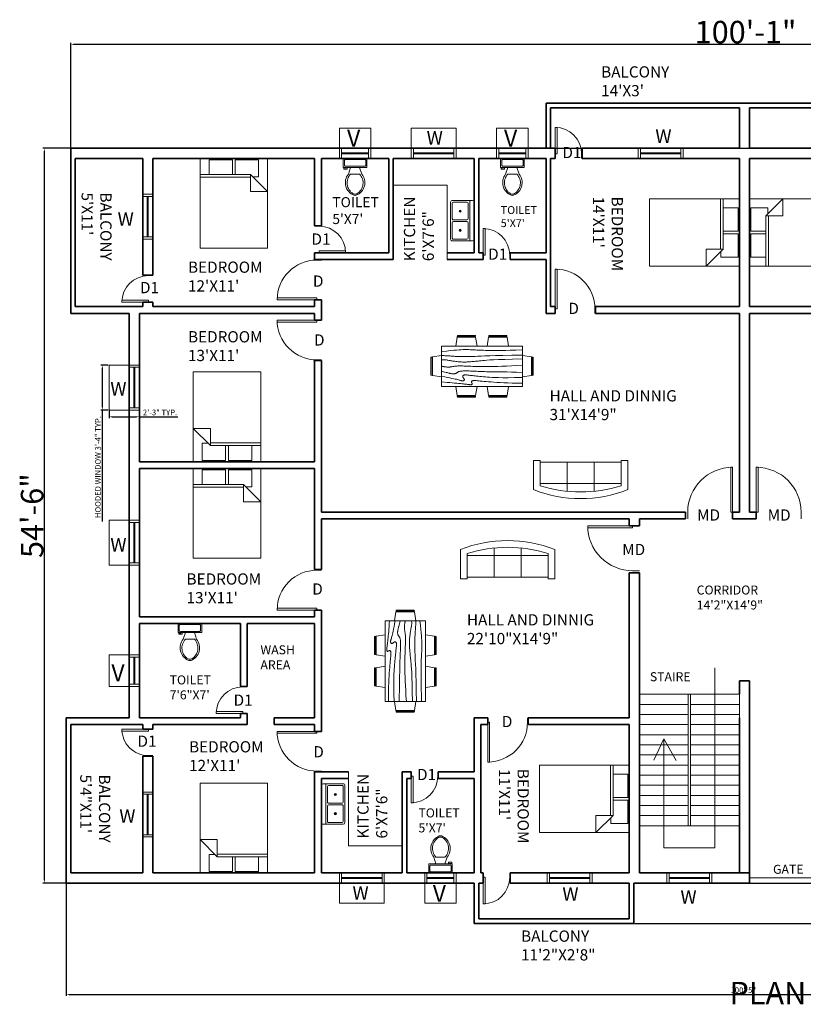
# Model space of a CAD drawing. Units: inches. Extents: x 1662 to 23131, y 1265 to 19127.
# Tile 18 of 26: x 19450 to 20147, y 18251 to 19127. Entities that reach past the tile are written whole.
import ezdxf

# ---------------------------------------------------------------- set-up
doc = ezdxf.new("R2010")
doc.units = ezdxf.units.IN
for name, color, linetype, lineweight in [('A-ANNO-DIMS', 4, 'Continuous', 18), ('A-ANNO-IDEN', 7, 'Continuous', 18), ('A-ANNO-TITL', 7, 'Continuous', 35), ('A-AREA-IDEN', 7, 'Continuous', 18), ('A-DOOR', 3, 'Continuous', 18), ('A-DOOR-GATE', 3, 'Continuous', 18), ('A-FLOR-CASE', 8, 'Continuous', 18), ('A-FLOR-FIXT', 9, 'Continuous', 18), ('A-FLOR-STRS', 7, 'Continuous', 18), ('A-FURN', 8, 'Continuous', 18), ('A-GLAZ', 4, 'Continuous', 18), ('A-WALL', 7, 'Continuous', 35)]:
    doc.layers.add(name, color=color, linetype=linetype, lineweight=lineweight)
doc.styles.get("Standard").update_dxf_attribs({"font": 'arial.ttf'})
doc.dimstyles.new('ISO-25', dxfattribs={"dimtxt": 5, "dimasz": 2.5, "dimexe": 1.25, "dimexo": 0.625, "dimtad": 1, "dimlunit": 3, "dimtxsty": 'Standard', "dimcen": 2.5, "dimadec": 0, "dimazin": 0, "dimtfac": 1, "dimtmove": 0, "dimatfit": 3, "dimfxl": 1, "dimarcsym": 0})

# ---------------------------------------------------------------- blocks, each defined once
blk = doc.blocks.new('Bed - Queen')
for p, q in [((0, -80.00003), (0, 0)), ((0, 0), (59.99999, 0)), ((59.99999, 0), (59.99999, -80.00003)), ((7.99999, -1.2), (28.79998, -1.2)), ((7.99999, -14.4), (7.99999, -1.2)), ((28.79998, -1.2), (28.79998, -14.4)), ((31.19999, -1.2), (51.99999, -1.2)), ((31.19999, -14.4), (31.19999, -1.2)), ((51.99999, -1.2), (51.99999, -16.4)), ((0, -14.4), (44.8, -14.4)), ((44.8, -16.8), (0, -16.8)), ((59.99999, -29.6), (44.8, -14.4)), ((44.8, -14.4), (44.8, -29.6)), ((51.99999, -16.4), (46.79936, -16.4)), ((44.8, -29.6), (59.99999, -29.6)), ((59.99999, -80.00003), (0, -80.00003))]:
    blk.add_line(p, q)
blk = doc.blocks.new('Toilet - top')
for p, q in [((-10, -8.5), (-8, -8.5)), ((-10, -9.5), (-10, -8.5)), ((-8, -8.5), (-8, -8)), ((-7, -8), (-7, -9.5)), ((-4, -8), (-6, -14)), ((4, -8), (6, -14)), ((9.5, -6), (9.5, -2)), ((-7, -9.5), (-10, -9.5)), ((4, -14), (-4, -14))]:
    blk.add_line(p, q)
blk.add_lwpolyline([(10.5, -8), (10.5, 0), (-10.5, 0), (-10.5, -8)], close=True)
for points in [[(-9.5, -2), (-9.5, -6)], [(8.5, -1), (-8.5, -1)], [(-8.5, -7), (8.5, -7)]]:
    blk.add_lwpolyline(points)
for centre, radius, start, end in [((-8.62, -1.88), 0.884, 81.8699, 188.1301), ((-8.62, -6.12), 0.884, 171.8699, 278.1301), ((8.62, -1.88), 0.884, 351.8699, 98.1301), ((8.62, -6.12), 0.884, 261.8699, 8.1301), ((3.52, -21.58), 12.17, 141.46911, 247.97143), ((4.2, -21.82), 11.33, 136.36773, 238.94682), ((-3.52, -21.58), 12.17, 292.02843, 38.53071), ((-4.2, -21.82), 11.33, 301.05301, 43.63209), ((0, -27.88), 4, 245.73182, 294.26817), ((0, -29), 4, 254.86053, 285.13947)]:
    blk.add_arc(centre, radius, start, end)
blk = doc.blocks.new('Sink-double - 36 in top')
for p, q in [((-18, -4), (18, -4)), ((-0.75, -18.5), (-0.75, -6.5)), ((0.75, -6.5), (0.75, -18.5))]:
    blk.add_line(p, q)
for points in [[(-16.5, 0), (16.5, 0)], [(-18, -19.5), (-18, -1.5)], [(-16.5, -18.5), (-16.5, -6.5)], [(-15.5, -5.5), (-1.75, -5.5)], [(1.75, -5.5), (15.5, -5.5)], [(16.5, -6.5), (16.5, -18.5)], [(18, -1.5), (18, -19.5)], [(16.5, -21), (-16.5, -21)], [(-1.75, -19.5), (-15.5, -19.5)], [(15.5, -19.5), (1.75, -19.5)]]:
    blk.add_lwpolyline(points)
for centre, radius in [((-8.5, -12.5), 1), ((-8.5, -12.5), 0.5), ((8.5, -12.5), 1), ((8.5, -12.5), 0.5)]:
    blk.add_circle(centre, radius)
for centre, radius, start, end in [((-16.5, -1.5), 1.5, 90, 180), ((16.5, -1.5), 1.5, 0, 90), ((-15.5, -6.5), 1, 90, 180), ((-1.75, -6.5), 1, 0, 90), ((1.75, -6.5), 1, 90, 180), ((15.5, -6.5), 1, 0, 90), ((-16.5, -19.5), 1.5, 180, 270), ((-15.5, -18.5), 1, 180, 270), ((-1.75, -18.5), 1, 270, 0), ((1.75, -18.5), 1, 180, 270), ((15.5, -18.5), 1, 270, 0), ((16.5, -19.5), 1.5, 270, 0)]:
    blk.add_arc(centre, radius, start, end)
blk = doc.blocks.new('Dining Set - 36 x 72 in.')
for p, q in [((-22, 27.5), (-22.1562, 26.50042)), ((-5.8416, 26.5), (-22.1534, 26.5)), ((-22, 27.5), (-6, 27.5)), ((-5.8437, 26.49966), (-6, 27.5)), ((6, 27.5), (5.8438, 26.50042)), ((22.1584, 26.5), (5.8466, 26.5)), ((6, 27.5), (22, 27.5)), ((22.1563, 26.49966), (22, 27.5)), ((36, 18), (-36, 18)), ((-36, 18), (-36, -18)), ((-22.2343, 26.00059), (-23.4847, 17.99762)), ((-22.2304, 26), (-5.7608, 26)), ((-4.5152, 17.99762), (-5.7655, 25.99926)), ((5.7657, 26.00059), (4.5153, 17.99762)), ((5.7696, 26), (22.2392, 26)), ((23.4848, 17.99762), (22.2345, 25.99926)), ((36, -18), (36, 18)), ((-44.0006, 8.23428), (-35.9976, 9.48474)), ((44.0006, 8.23428), (35.9976, 9.48474)), ((-45.5, 8), (-44.5004, 8.15617)), ((-45.5, 8), (-45.5, -8)), ((-44.5, -8.15843), (-44.5, 8.15338)), ((-44, 8.23041), (-44, -8.23915)), ((44, 8.23041), (44, -8.23915)), ((44.5, -8.15843), (44.5, 8.15338)), ((45.5, 8), (44.5005, 8.15617)), ((45.5, 8), (45.5, -8)), ((-44.4997, -8.15631), (-45.5, -8)), ((-35.9976, -9.48476), (-43.9993, -8.2345)), ((35.9976, -9.48476), (43.9993, -8.2345)), ((44.4997, -8.15631), (45.5, -8)), ((-36, -18), (36, -18)), ((-22.2343, -26.0006), (-23.4847, -17.99762)), ((-22.2304, -26), (-5.7608, -26)), ((-4.5152, -17.99762), (-5.7655, -25.99928)), ((5.7657, -26.0006), (4.5153, -17.99762)), ((5.7696, -26), (22.2392, -26)), ((23.4848, -17.99762), (22.2345, -25.99928)), ((-22, -27.5), (-22.1562, -26.50044)), ((-5.8416, -26.5), (-22.1534, -26.5)), ((-22, -27.5), (-6, -27.5)), ((-5.8437, -26.49967), (-6, -27.5)), ((6, -27.5), (5.8438, -26.50044)), ((22.1584, -26.5), (5.8466, -26.5)), ((6, -27.5), (22, -27.5)), ((22.1563, -26.49967), (22, -27.5))]:
    blk.add_line(p, q)
for points in [[(-36, 15), (-31.1772, 14.97754), (-26.8079, 14.91406), (-22.8538, 14.81543), (-19.276, 14.6875), (-16.0362, 14.53613), (-13.0957, 14.36718), (-10.4159, 14.18652), (-7.9583, 14), (-5.6904, 13.81315), (-3.6035, 13.63021), (-1.6954, 13.45508), (0.0365, 13.29166), (1.5945, 13.14388), (2.9811, 13.01562), (4.1988, 12.9108), (5.25, 12.83333), (6.1393, 12.78613), (6.8802, 12.76823), (7.4883, 12.77767), (7.9792, 12.8125), (8.3685, 12.87077), (8.6719, 12.95052), (8.9049, 13.0498), (9.0833, 13.16666), (9.2205, 13.29899), (9.3216, 13.44401), (9.3895, 13.59879), (9.4271, 13.76041), (9.4373, 13.92594), (9.4232, 14.09245), (9.3875, 14.257), (9.3333, 14.41666), (9.2638, 14.56917), (9.1836, 14.71484), (9.0975, 14.85465), (9.0104, 14.98958), (8.9272, 15.1206), (8.8529, 15.2487), (8.7922, 15.37483), (8.75, 15.5), (8.7305, 15.62467), (8.7344, 15.74739), (8.7617, 15.86621), (8.8125, 15.97916), (8.8867, 16.08431), (8.9844, 16.17968), (9.1055, 16.26334), (9.25, 16.33333), (9.4189, 16.38802), (9.6172, 16.42708), (9.8506, 16.45052), (10.125, 16.45833), (10.4463, 16.45052), (10.8203, 16.42708), (11.2529, 16.38802), (11.75, 16.33333), (12.3184, 16.26318), (12.9694, 16.17838), (13.7151, 16.07991), (14.5677, 15.96875), (15.5395, 15.84586), (16.6426, 15.71224), (17.8893, 15.56884), (19.2917, 15.41666), (20.859, 15.25667), (22.5879, 15.08984), (24.4721, 14.91715), (26.5052, 14.73958), (28.6809, 14.5581), (30.9929, 14.3737), (33.4347, 14.18733), (36, 14)], [(-36, 10), (-28.9766, 10.14274), (-23.1725, 10.20442), (-18.4241, 10.19775), (-14.5677, 10.13541), (-11.4399, 10.03011), (-8.877, 9.89453), (-6.7154, 9.74137), (-4.7917, 9.58333), (-2.9698, 9.43082), (-1.2246, 9.28515), (0.4415, 9.14534), (2.026, 9.01041), (3.5266, 8.87939), (4.9408, 8.7513), (6.266, 8.62516), (7.5, 8.5), (8.6411, 8.37549), (9.6914, 8.2539), (10.6538, 8.13818), (11.5312, 8.03125), (12.3267, 7.93603), (13.043, 7.85547), (13.6831, 7.79248), (14.25, 7.75), (14.7471, 7.7303), (15.1797, 7.73307), (15.5537, 7.75732), (15.875, 7.80208), (16.1494, 7.86637), (16.3828, 7.94922), (16.5811, 8.04964), (16.75, 8.16666), (16.8944, 8.29915), (17.0143, 8.44531), (17.1089, 8.60319), (17.1771, 8.77083), (17.218, 8.94629), (17.2305, 9.1276), (17.2137, 9.31282), (17.1667, 9.5), (17.0895, 9.6875), (16.987, 9.875), (16.8649, 10.0625), (16.7292, 10.25), (16.5856, 10.4375), (16.4401, 10.625), (16.2985, 10.8125), (16.1667, 11), (16.05, 11.18733), (15.9518, 11.3737), (15.8752, 11.5581), (15.8229, 11.73958), (15.798, 11.91715), (15.8034, 12.08984), (15.842, 12.25667), (15.9167, 12.41666), (16.0295, 12.56836), (16.1784, 12.70833), (16.3605, 12.83268), (16.5729, 12.9375), (16.8127, 13.01888), (17.0768, 13.07291), (17.3625, 13.0957), (17.6667, 13.08333), (17.9894, 13.03312), (18.3418, 12.94726), (18.7382, 12.82918), (19.1927, 12.68229), (19.7195, 12.51001), (20.3327, 12.31575), (21.0465, 12.10294), (21.875, 11.875), (22.8357, 11.63354), (23.959, 11.37304), (25.2786, 11.08618), (26.8282, 10.76562), (28.6414, 10.40405), (30.752, 9.99414), (33.1936, 9.52856), (36, 9)], [(-36, 5.5), (-30.7157, 5.3348), (-26.069, 5.20963), (-21.9946, 5.11767), (-18.4271, 5.05208), (-15.3009, 5.00602), (-12.5508, 4.97265), (-10.1112, 4.94515), (-7.9167, 4.91666), (-5.909, 4.88167), (-4.0586, 4.83984), (-2.3429, 4.79215), (-0.7396, 4.73958), (0.7739, 4.6831), (2.22, 4.6237), (3.6213, 4.56233), (5, 4.5), (6.373, 4.43782), (7.7344, 4.3776), (9.0723, 4.32129), (10.375, 4.27083), (11.6309, 4.22819), (12.8281, 4.19531), (13.9551, 4.17415), (15, 4.16666), (15.954, 4.17448), (16.819, 4.19791), (17.6001, 4.23698), (18.3021, 4.29166), (18.9299, 4.36198), (19.4883, 4.44791), (19.9823, 4.54948), (20.4167, 4.66666), (20.7969, 4.79899), (21.1302, 4.94401), (21.4245, 5.09879), (21.6875, 5.26041), (21.9271, 5.42594), (22.1511, 5.59245), (22.3672, 5.757), (22.5834, 5.91666), (22.8065, 6.06868), (23.0404, 6.21093), (23.2879, 6.34147), (23.5521, 6.45833), (23.8358, 6.55957), (24.142, 6.64323), (24.4735, 6.70735), (24.8334, 6.75), (25.2235, 6.76969), (25.642, 6.76692), (26.0858, 6.74267), (26.5521, 6.69791), (27.0379, 6.63362), (27.5404, 6.55078), (28.0565, 6.45036), (28.5834, 6.33333), (29.1242, 6.19987), (29.7071, 6.04687), (30.3661, 5.87044), (31.1354, 5.66666), (32.0493, 5.43164), (33.142, 5.16146), (34.4475, 4.85221), (36, 4.5)], [(-36, -1), (-30.7915, -0.6591), (-26.0195, -0.38216), (-21.6519, -0.16284), (-17.6563, 0.00521), (-14.0005, 0.12833), (-10.6523, 0.21289), (-7.5796, 0.26522), (-4.75, 0.29166), (-2.134, 0.29793), (0.2878, 0.28711), (2.5317, 0.26163), (4.6146, 0.22396), (6.5529, 0.17651), (8.3633, 0.12174), (10.0623, 0.06209), (11.6667, 0), (13.1899, -0.06201), (14.6341, -0.1211), (15.9982, -0.17432), (17.2813, -0.21875), (18.4823, -0.25147), (19.6003, -0.26953), (20.6343, -0.27002), (21.5834, -0.25), (22.4481, -0.20768), (23.2357, -0.14584), (23.9549, -0.06836), (24.6146, 0.02083), (25.2235, 0.11784), (25.7904, 0.21875), (26.3241, 0.31966), (26.8334, 0.41666), (27.3265, 0.50618), (27.8099, 0.58593), (28.2894, 0.65397), (28.7709, 0.70833), (29.2601, 0.74707), (29.763, 0.76823), (30.2855, 0.76985), (30.8334, 0.75), (31.4088, 0.70784), (31.9994, 0.64713), (32.589, 0.57275), (33.1615, 0.48958), (33.7008, 0.4025), (34.1908, 0.3164), (34.6153, 0.23616), (34.9584, 0.16666), (35.2099, 0.11165), (35.3848, 0.07031), (35.504, 0.04069), (35.5886, 0.02083), (35.6594, 0.00879), (35.7377, 0.0026), (35.8442, 0.00032), (36, 0)], [(-36, -6.5), (-27.1843, -6.31267), (-20.084, -6.1263), (-14.469, -5.9419), (-10.1094, -5.76042), (-6.7752, -5.58285), (-4.2363, -5.41016), (-2.2629, -5.24333), (-0.625, -5.08334), (0.8708, -4.93099), (2.2715, -4.78646), (3.5872, -4.64974), (4.8281, -4.52084), (6.0046, -4.39974), (7.127, -4.28646), (8.2053, -4.18099), (9.25, -4.08334), (10.2705, -3.99382), (11.2734, -3.91407), (12.2647, -3.84603), (13.25, -3.79167), (14.2354, -3.75293), (15.2266, -3.73177), (16.2295, -3.73015), (17.25, -3.75), (18.2912, -3.79248), (19.3451, -3.85547), (20.4009, -3.93604), (21.4479, -4.03125), (22.4754, -4.13819), (23.4727, -4.25391), (24.4289, -4.37549), (25.3334, -4.5), (26.1785, -4.62492), (26.9694, -4.74935), (27.7145, -4.87281), (28.4219, -4.99479), (29.1, -5.11483), (29.7572, -5.23242), (30.4016, -5.34709), (31.0417, -5.45834), (31.6837, -5.56437), (32.3262, -5.65821), (32.9658, -5.73153), (33.599, -5.77604), (34.2224, -5.78345), (34.8327, -5.74545), (35.4264, -5.65373), (36, -5.5)], [(-36, -10), (-26.4022, -9.81299), (-18.4675, -9.62891), (-11.9839, -9.45069), (-6.7396, -9.28125), (-2.5226, -9.12354), (0.8789, -8.98047), (3.6769, -8.85498), (6.0833, -8.75), (8.2767, -8.66765), (10.3021, -8.60677), (12.1712, -8.56543), (13.8958, -8.54167), (15.4876, -8.53353), (16.9583, -8.53907), (18.3197, -8.55632), (19.5834, -8.58334), (20.7616, -8.61841), (21.8685, -8.66081), (22.9188, -8.71004), (23.9271, -8.76563), (24.9081, -8.82707), (25.8763, -8.89388), (26.8465, -8.96558), (27.8334, -9.04167), (28.8474, -9.12118), (29.8828, -9.20117), (30.93, -9.27824), (31.9792, -9.34896), (33.0205, -9.40991), (34.0443, -9.45768), (35.0407, -9.48885), (36, -9.5)], [(-36, -14.5), (-30.0881, -14.33513), (-25.0332, -14.21224), (-20.7312, -14.12647), (-17.0781, -14.07292), (-13.97, -14.04671), (-11.3027, -14.04297), (-8.9724, -14.05681), (-6.875, -14.08334), (-4.9224, -14.11833), (-3.0905, -14.16016), (-1.3709, -14.20785), (0.2448, -14.26042), (1.7647, -14.3169), (3.1973, -14.3763), (4.5507, -14.43767), (5.8333, -14.5), (7.0554, -14.5621), (8.235, -14.62175), (9.3922, -14.67652), (10.5469, -14.72396), (11.7192, -14.76164), (12.929, -14.78711), (14.1965, -14.79794), (15.5417, -14.79167), (16.9933, -14.76424), (18.6152, -14.70508), (20.4804, -14.60197), (22.6615, -14.44271), (25.2312, -14.21509), (28.2624, -13.9069), (31.8277, -13.50594), (36, -13)]]:
    blk.add_lwpolyline(points)
blk = doc.blocks.new('Sofa - Roundback 7 ft.')
for p, q in [((-12.00002, -32.4421), (-12.00003, -6.5971)), ((11.99997, -32.4421), (11.99998, -6.5971)), ((-36.000027, -34), (-36.000027, -11.4696)), ((-35.999844, -13.3819), (35.9998, -13.3819)), ((35.99998, -34), (35.99998, -11.4696)), ((-36.000027, -32.4421), (35.99998, -32.4421))]:
    blk.add_line(p, q)
for points in [[(-36.000027, -34), (-42.000027, -34), (-42.000027, -8)], [(41.99998, -8), (41.99998, -34), (35.99998, -34)]]:
    blk.add_lwpolyline(points)
for centre, radius, start, end in [((0, -114.25), 114.25, 68.43141, 111.5686), ((-0.00001, -127.1968), 121.1968, 72.72033, 107.2797)]:
    blk.add_arc(centre, radius, start, end)
blk = doc.blocks.new('*U26')
for p, q in [((0, 0), (0, -100)), ((900, 0), (900, -100))]:
    blk.add_line(p, q)
blk.add_lwpolyline([(0, 0), (0, 900), (43.75, 900), (43.75, 0)], close=True)
blk.add_arc((0, 0), 900, 0, 90)
blk = doc.blocks.new('*U99')
for p, q in [((0, 0), (0, 100)), ((900, 0), (900, 100))]:
    blk.add_line(p, q)
blk.add_lwpolyline([(0, 0), (0, -900), (43.75, -900), (43.75, 0)], close=True)
blk.add_arc((0, 0), 900, 270, 0)
blk = doc.blocks.new('*U102')
for p, q in [((0, 0), (0, 100)), ((900, 0), (900, 100))]:
    blk.add_line(p, q)
blk.add_lwpolyline([(0, 0), (0, -900), (43.75, -900), (43.75, 0)], close=True)
blk.add_arc((0, 0), 900, 270, 0)
blk = doc.blocks.new('*U100')
for p, q in [((-900, 0), (-900, 100)), ((0, 0), (0, 100))]:
    blk.add_line(p, q)
blk.add_lwpolyline([(0, 0), (0, -900), (-43.75, -900), (-43.75, 0)], close=True)
blk.add_arc((0, 0), 900, 180, 270)
blk = doc.blocks.new('*U109')
for p, q in [((0, 0), (0, 100)), ((600, 0), (600, 100))]:
    blk.add_line(p, q)
blk.add_lwpolyline([(0, 0), (0, -600), (43.75, -600), (43.75, 0)], close=True)
blk.add_arc((0, 0), 600, 270, 0)
blk = doc.blocks.new('*U110')
for p, q in [((-600, 0), (-600, 100)), ((0, 0), (0, 100))]:
    blk.add_line(p, q)
blk.add_lwpolyline([(0, 0), (0, -600), (-43.75, -600), (-43.75, 0)], close=True)
blk.add_arc((0, 0), 600, 180, 270)
blk = doc.blocks.new('*U105')
for p, q in [((-600, 0), (-600, -100)), ((0, 0), (0, -100))]:
    blk.add_line(p, q)
blk.add_lwpolyline([(0, 0), (0, 600), (-43.75, 600), (-43.75, 0)], close=True)
blk.add_arc((0, 0), 600, 90, 180)
blk = doc.blocks.new('*U112')
for p, q in [((-600, 0), (-600, 100)), ((0, 0), (0, 100))]:
    blk.add_line(p, q)
blk.add_lwpolyline([(0, 0), (0, -600), (-43.75, -600), (-43.75, 0)], close=True)
blk.add_arc((0, 0), 600, 180, 270)
blk = doc.blocks.new('*U111')
for p, q in [((0, 0), (0, 100)), ((600, 0), (600, 100))]:
    blk.add_line(p, q)
blk.add_lwpolyline([(0, 0), (0, -600), (43.75, -600), (43.75, 0)], close=True)
blk.add_arc((0, 0), 600, 270, 0)
blk = doc.blocks.new('*U10')
for p, q in [((0, 0), (0, -6)), ((40, 0), (40, -6))]:
    blk.add_line(p, q)
blk.add_lwpolyline([(0, 0), (0, 40), (1.75, 40), (1.75, 0)], close=True)
blk.add_arc((0, 0), 40, 0, 90)
blk = doc.blocks.new('*U27')
for p, q in [((0, 0), (0, -6)), ((-40, 0), (-40, -6))]:
    blk.add_line(p, q)
blk.add_lwpolyline([(0, 0), (0, 40), (-1.75, 40), (-1.75, 0)], close=True)
blk.add_arc((0, 0), 40, 90, 180)
blk = doc.blocks.new('*U114')
for p, q in [((0, 0), (0, 6)), ((40, 0), (40, 6))]:
    blk.add_line(p, q)
blk.add_lwpolyline([(0, 0), (0, -40), (1.75, -40), (1.75, 0)], close=True)
blk.add_arc((0, 0), 40, 270, 0)
blk = doc.blocks.new('*U106')
for p, q in [((-600, 0), (-600, 100)), ((0, 0), (0, 100))]:
    blk.add_line(p, q)
blk.add_lwpolyline([(0, 0), (0, -600), (-43.75, -600), (-43.75, 0)], close=True)
blk.add_arc((0, 0), 600, 180, 270)
blk = doc.blocks.new('*D115')
at = {"layer": 'A-ANNO-DIMS', "color": 0, "lineweight": -2, "transparency": 16777216}
for p, q in [((19495.19, 19013.32), (19495.19, 19106.49)), ((19497.69, 19105.24), (20693.69, 19105.24)), ((20696.19, 19013.32), (20696.19, 19106.49))]:
    blk.add_line(p, q, dxfattribs=at)
at = {"layer": 'A-ANNO-DIMS', "color": 0, "transparency": 16777216}
for points in [[(19497.69, 19105.65), (19497.69, 19104.82), (19495.19, 19105.24)], [(20693.69, 19105.65), (20693.69, 19104.82), (20696.19, 19105.24)]]:
    blk.add_solid(points, dxfattribs=at)
at = {"layer": 'Defpoints', "color": 0, "transparency": 16777216}
for p in [(20696.19, 19105.24), (19495.19, 19012.7), (20696.19, 19012.7)]:
    blk.add_point(p, dxfattribs=at)
at = {"layer": 'A-ANNO-DIMS', "color": 0, "transparency": 16777216, "insert": (20095.69, 19116.07), "char_height": 5, "attachment_point": 5}
blk.add_mtext('{\\H4x;100\'-1"}', dxfattribs=at)
blk = doc.blocks.new('*D116')
at = {"layer": 'A-ANNO-DIMS', "color": 0, "lineweight": -2, "transparency": 16777216}
for p, q in [((19494.57, 19012.7), (19470.34, 19012.7)), ((19471.59, 19010.2), (19471.59, 18361.2)), ((19494.57, 18358.7), (19470.34, 18358.7))]:
    blk.add_line(p, q, dxfattribs=at)
at = {"layer": 'A-ANNO-DIMS', "color": 0, "transparency": 16777216}
for points in [[(19471.17, 19010.2), (19472, 19010.2), (19471.59, 19012.7)], [(19471.17, 18361.2), (19472, 18361.2), (19471.59, 18358.7)]]:
    blk.add_solid(points, dxfattribs=at)
at = {"layer": 'Defpoints', "color": 0, "transparency": 16777216}
for p in [(19495.19, 19012.7), (19471.59, 18358.7), (19495.19, 18358.7)]:
    blk.add_point(p, dxfattribs=at)
at = {"layer": 'A-ANNO-DIMS', "color": 0, "transparency": 16777216, "insert": (19460.75, 18685.7), "char_height": 5, "attachment_point": 5, "rotation": 90}
blk.add_mtext('{\\H4x;54\'-6"}', dxfattribs=at)
blk = doc.blocks.new('WIN-36-J9X2')
for p, q in [((0, 0), (0, 9)), ((2, 0), (2, 9)), ((38, 0), (38, 9)), ((40, 0), (40, 9)), ((38, 5), (2, 5)), ((38, 4.5), (2, 4.5)), ((38, 4), (2, 4))]:
    blk.add_line(p, q)
blk = doc.blocks.new('WIN-36-J9X2-HOOD')
for p, q in [((0, 27), (0, 18)), ((2, 27), (2, 18)), ((38, 27), (38, 18)), ((40, 27), (40, 18)), ((0, 18), (0, 0)), ((2, 23), (38, 23)), ((2, 22.5), (38, 22.5)), ((2, 22), (38, 22)), ((40, 0), (40, 18)), ((0, 0), (40, 0))]:
    blk.add_line(p, q)
blk = doc.blocks.new('VENT-24-J9X2-HOOD')
for p, q in [((0, 18), (0, 27)), ((2, 18), (2, 27)), ((26, 18), (26, 27)), ((28, 18), (28, 27)), ((0, 18), (0, 0)), ((26, 23), (2, 23)), ((26, 22.5), (2, 22.5)), ((26, 22), (2, 22)), ((28, 0), (28, 18)), ((0, 0), (28, 0))]:
    blk.add_line(p, q)
blk = doc.blocks.new('*D173')
at = {"layer": 'A-ANNO-DIMS', "color": 0, "lineweight": -2, "transparency": 16777216}
for p, q in [((19528.57, 18819.7), (19521.94, 18819.7)), ((19523.19, 18817.2), (19523.19, 18782.2)), ((19528.57, 18779.7), (19521.94, 18779.7)), ((19523.19, 18779.7), (19523.19, 18680.55))]:
    blk.add_line(p, q, dxfattribs=at)
at = {"layer": 'A-ANNO-DIMS', "color": 0, "transparency": 16777216}
for points in [[(19522.78, 18817.2), (19523.61, 18817.2), (19523.19, 18819.7)], [(19522.78, 18782.2), (19523.61, 18782.2), (19523.19, 18779.7)]]:
    blk.add_solid(points, dxfattribs=at)
at = {"layer": 'Defpoints', "color": 0, "transparency": 16777216}
for p in [(19529.19, 18819.7), (19523.19, 18779.7), (19529.19, 18779.7)]:
    blk.add_point(p, dxfattribs=at)
at = {"layer": 'A-ANNO-DIMS', "color": 0, "transparency": 16777216, "insert": (19519.98, 18728.87), "char_height": 5, "attachment_point": 5, "rotation": 90}
blk.add_mtext('HOODED WINDOW 3\'-4" TYP.', dxfattribs=at)
blk = doc.blocks.new('*D174')
at = {"layer": 'A-ANNO-DIMS', "color": 0, "lineweight": -2, "transparency": 16777216}
for p, q in [((19529.19, 18779.07), (19529.19, 18772.45)), ((19531.69, 18773.7), (19553.69, 18773.7)), ((19556.19, 18779.07), (19556.19, 18772.45)), ((19556.19, 18773.7), (19590.51, 18773.7))]:
    blk.add_line(p, q, dxfattribs=at)
at = {"layer": 'A-ANNO-DIMS', "color": 0, "transparency": 16777216}
for points in [[(19531.69, 18774.11), (19531.69, 18773.28), (19529.19, 18773.7)], [(19553.69, 18774.11), (19553.69, 18773.28), (19556.19, 18773.7)]]:
    blk.add_solid(points, dxfattribs=at)
at = {"layer": 'Defpoints', "color": 0, "transparency": 16777216}
for p in [(19529.19, 18779.7), (19556.19, 18779.7), (19556.19, 18773.7)]:
    blk.add_point(p, dxfattribs=at)
at = {"layer": 'A-ANNO-DIMS', "color": 0, "transparency": 16777216, "insert": (19574.6, 18776.88), "char_height": 5, "attachment_point": 5}
blk.add_mtext('2\'-3" TYP.', dxfattribs=at)
blk = doc.blocks.new('*D251')
at = {"layer": 'A-ANNO-DIMS', "color": 0, "lineweight": -2, "transparency": 16777216}
for p, q in [((19491.19, 18358.07), (19491.19, 18258.3)), ((20696.19, 18358.07), (20696.19, 18258.3)), ((19493.69, 18259.55), (20693.69, 18259.55))]:
    blk.add_line(p, q, dxfattribs=at)
at = {"layer": 'A-ANNO-DIMS', "color": 0, "transparency": 16777216}
for points in [[(19493.69, 18259.96), (19493.69, 18259.13), (19491.19, 18259.55)], [(20693.69, 18259.96), (20693.69, 18259.13), (20696.19, 18259.55)]]:
    blk.add_solid(points, dxfattribs=at)
at = {"layer": 'Defpoints', "color": 0, "transparency": 16777216}
for p in [(19491.19, 18358.7), (20696.19, 18358.7), (20696.19, 18259.55)]:
    blk.add_point(p, dxfattribs=at)
at = {"layer": 'A-ANNO-DIMS', "color": 0, "transparency": 16777216, "insert": (20093.69, 18262.72), "char_height": 5, "attachment_point": 5}
blk.add_mtext('100\'-5"', dxfattribs=at)
blk = doc.blocks.new('*D252')
at = {"layer": 'A-ANNO-DIMS', "color": 0, "lineweight": -2, "transparency": 16777216}
for p, q in [((19918.82, 19052.7), (20760.59, 19052.7)), ((20759.34, 19015.2), (20759.34, 19050.2)), ((19918.82, 19012.7), (20760.59, 19012.7))]:
    blk.add_line(p, q, dxfattribs=at)
at = {"layer": 'A-ANNO-DIMS', "color": 0, "transparency": 16777216}
for points in [[(20758.93, 19050.2), (20759.76, 19050.2), (20759.34, 19052.7)], [(20758.93, 19015.2), (20759.76, 19015.2), (20759.34, 19012.7)]]:
    blk.add_solid(points, dxfattribs=at)
at = {"layer": 'Defpoints', "color": 0, "transparency": 16777216}
for p in [(19918.19, 19052.7), (20759.34, 19052.7), (19918.19, 19012.7)]:
    blk.add_point(p, dxfattribs=at)
at = {"layer": 'A-ANNO-DIMS', "color": 0, "transparency": 16777216, "insert": (20756.16, 19032.7), "char_height": 5, "attachment_point": 5, "rotation": 90}
blk.add_mtext('3\'-4"', dxfattribs=at)
blk = doc.blocks.new('*D253')
at = {"layer": 'A-ANNO-DIMS', "color": 0, "lineweight": -2, "transparency": 16777216}
for p, q in [((19996.82, 18358.7), (20760.59, 18358.7)), ((20759.34, 18325.2), (20759.34, 18356.2)), ((19996.82, 18322.7), (20760.59, 18322.7))]:
    blk.add_line(p, q, dxfattribs=at)
at = {"layer": 'A-ANNO-DIMS', "color": 0, "transparency": 16777216}
for points in [[(20758.93, 18356.2), (20759.76, 18356.2), (20759.34, 18358.7)], [(20758.93, 18325.2), (20759.76, 18325.2), (20759.34, 18322.7)]]:
    blk.add_solid(points, dxfattribs=at)
at = {"layer": 'Defpoints', "color": 0, "transparency": 16777216}
for p in [(19996.19, 18358.7), (20759.34, 18358.7), (19996.19, 18322.7)]:
    blk.add_point(p, dxfattribs=at)
at = {"layer": 'A-ANNO-DIMS', "color": 0, "transparency": 16777216, "insert": (20756.16, 18340.7), "char_height": 5, "attachment_point": 5, "rotation": 90}
blk.add_mtext('3\'-0"', dxfattribs=at)

msp = doc.modelspace()

# ---------------------------------------------------------------- linework, layer by layer
at = {"layer": 'A-DOOR-GATE'}
msp.add_line((20099.192, 18363.196), (20168.192, 18363.196), dxfattribs=at)
at = {"layer": 'A-FLOR-CASE'}
for p, q in [((19782.192, 18979.696), (19830.192, 18979.696)), ((19830.192, 18913.696), (19830.192, 18979.696)), ((19742.192, 18391.696), (19742.192, 18457.696)), ((19742.192, 18391.696), (19790.192, 18391.696))]:
    msp.add_line(p, q, dxfattribs=at)
at = {"layer": 'A-FLOR-STRS'}
for p, q in [((20068.442, 18550.107), (20068.442, 18390.107)), ((20001.192, 18526.696), (20090.192, 18526.696)), ((20044.692, 18409.696), (20044.692, 18526.696)), ((20046.692, 18409.696), (20046.692, 18526.696)), ((20090.192, 18505.696), (20090.192, 18526.696)), ((20001.192, 18517.696), (20044.692, 18517.696)), ((20046.692, 18517.696), (20090.192, 18517.696)), ((20001.192, 18508.696), (20044.692, 18508.696)), ((20046.692, 18508.696), (20090.192, 18508.696)), ((20001.192, 18499.696), (20044.692, 18499.696)), ((20046.692, 18499.696), (20090.192, 18499.696)), ((20001.192, 18490.696), (20044.692, 18490.696)), ((20022.942, 18486.908), (20013.925, 18467.991)), ((20022.942, 18390.107), (20022.942, 18486.908)), ((20022.942, 18486.908), (20033.987, 18467.711)), ((20046.692, 18490.696), (20090.192, 18490.696)), ((20001.192, 18481.696), (20044.692, 18481.696)), ((20046.692, 18481.696), (20090.192, 18481.696)), ((20001.192, 18472.696), (20044.692, 18472.696)), ((20046.692, 18472.696), (20090.192, 18472.696)), ((20001.192, 18463.696), (20044.692, 18463.696)), ((20046.692, 18463.696), (20090.192, 18463.696)), ((20001.192, 18454.696), (20044.692, 18454.696)), ((20046.692, 18454.696), (20090.192, 18454.696)), ((20001.192, 18445.696), (20044.692, 18445.696)), ((20046.692, 18445.696), (20090.192, 18445.696)), ((20001.192, 18436.696), (20044.692, 18436.696)), ((20046.692, 18436.696), (20090.192, 18436.696)), ((20001.192, 18427.696), (20044.692, 18427.696)), ((20046.692, 18427.696), (20090.192, 18427.696)), ((20001.192, 18418.696), (20044.692, 18418.696)), ((20046.692, 18418.696), (20090.192, 18418.696)), ((20001.192, 18409.696), (20090.192, 18409.696)), ((20068.442, 18390.107), (20022.942, 18390.107))]:
    msp.add_line(p, q, dxfattribs=at)
at = {"layer": 'A-WALL'}
for p, q in [((19918.192, 19012.696), (19918.192, 19052.696)), ((19918.192, 19052.696), (20271.192, 19052.696)), ((19922.192, 19012.696), (19922.192, 19048.696)), ((19922.192, 19048.696), (20090.192, 19048.696)), ((20090.192, 19012.696), (20090.192, 19048.696)), ((20099.192, 19012.696), (20099.192, 19048.696)), ((20099.192, 19048.696), (20267.192, 19048.696)), ((19495.192, 18865.696), (19495.192, 19012.696)), ((19495.192, 19012.696), (19926.192, 19012.696)), ((19926.192, 19003.696), (19926.192, 19012.696)), ((19950.192, 19003.696), (19950.192, 19012.696)), ((19950.192, 19012.696), (20090.192, 19012.696)), ((20099.192, 19012.696), (20239.192, 19012.696)), ((19499.192, 19003.696), (19559.192, 19003.696)), ((19499.192, 18871.696), (19499.192, 19003.696)), ((19559.192, 18899.696), (19559.192, 19003.696)), ((19568.192, 18899.696), (19568.192, 19003.696)), ((19568.192, 19003.696), (19712.192, 19003.696)), ((19712.192, 18943.696), (19712.192, 19003.696)), ((19718.192, 18943.696), (19718.192, 19003.696)), ((19718.192, 19003.696), (19778.192, 19003.696)), ((19778.192, 18919.696), (19778.192, 19003.696)), ((19782.192, 18913.696), (19782.192, 19003.696)), ((19782.192, 19003.696), (19854.192, 19003.696)), ((19854.192, 18919.696), (19854.192, 19003.696)), ((19858.192, 18919.696), (19858.192, 19003.696)), ((19858.192, 19003.696), (19918.192, 19003.696)), ((19918.192, 18919.696), (19918.192, 19003.696)), ((19922.192, 18871.696), (19922.192, 19003.696)), ((19922.192, 19003.696), (19926.192, 19003.696)), ((19950.192, 19003.696), (20090.192, 19003.696)), ((20090.192, 18871.696), (20090.192, 19003.696)), ((20099.192, 19003.696), (20239.192, 19003.696)), ((20099.192, 18871.696), (20099.192, 19003.696)), ((19854.192, 18948.185), (19854.192, 18948.185)), ((19712.192, 18943.696), (19718.192, 18943.696)), ((19712.192, 18919.696), (19778.192, 18919.696)), ((19712.192, 18913.696), (19712.192, 18919.696)), ((19712.192, 18913.696), (19782.192, 18913.696)), ((19830.192, 18919.696), (19854.192, 18919.696)), ((19830.192, 18913.696), (19862.192, 18913.696)), ((19858.192, 18919.696), (19862.192, 18919.696)), ((19862.192, 18913.696), (19862.192, 18919.696)), ((19886.192, 18913.696), (19886.192, 18919.696)), ((19886.192, 18919.696), (19918.192, 18919.696)), ((19886.192, 18913.696), (19918.192, 18913.696)), ((19918.192, 18865.696), (19918.192, 18913.696)), ((19559.192, 18899.696), (19568.192, 18899.696)), ((19712.192, 18877.696), (19718.192, 18877.696)), ((19712.192, 18871.696), (19712.192, 18877.696)), ((19718.192, 18859.696), (19718.192, 18877.696)), ((19499.192, 18871.696), (19559.192, 18871.696)), ((19559.192, 18871.696), (19559.192, 18875.696)), ((19559.192, 18875.696), (19568.192, 18875.696)), ((19568.192, 18871.696), (19568.192, 18875.696)), ((19568.192, 18871.696), (19712.192, 18871.696)), ((19922.192, 18871.696), (19926.192, 18871.696)), ((19926.192, 18865.696), (19926.192, 18871.696)), ((19962.192, 18865.696), (19962.192, 18871.696)), ((19962.192, 18871.696), (20090.192, 18871.696)), ((20099.192, 18871.696), (20227.192, 18871.696)), ((19495.192, 18865.696), (19547.192, 18865.696)), ((19547.192, 18505.696), (19547.192, 18865.696)), ((19556.192, 18865.696), (19712.192, 18865.696)), ((19556.192, 18733.696), (19556.192, 18865.696)), ((19712.192, 18859.696), (19712.192, 18865.696)), ((19718.192, 18859.696), (19712.192, 18859.696)), ((19918.192, 18865.696), (19926.192, 18865.696)), ((19962.192, 18865.696), (20090.192, 18865.696)), ((20090.192, 18688.696), (20090.192, 18865.696)), ((20099.192, 18688.696), (20099.192, 18865.696)), ((20099.192, 18865.696), (20227.192, 18865.696)), ((19718.192, 18823.696), (19712.192, 18823.696)), ((19712.192, 18733.696), (19712.192, 18823.696)), ((19718.192, 18688.696), (19718.192, 18823.696)), ((19556.192, 18733.696), (19712.192, 18733.696)), ((19556.192, 18727.696), (19712.192, 18727.696)), ((19556.192, 18595.696), (19556.192, 18727.696)), ((19712.192, 18637.696), (19712.192, 18727.696)), ((19718.192, 18688.696), (20042.192, 18688.696)), ((20042.192, 18682.696), (20042.192, 18688.696)), ((20084.192, 18682.696), (20084.192, 18688.696)), ((20084.192, 18688.696), (20090.192, 18688.696)), ((20099.192, 18688.696), (20105.192, 18688.696)), ((20105.192, 18682.696), (20105.192, 18688.696)), ((19718.192, 18682.696), (19992.192, 18682.696)), ((19718.192, 18637.696), (19718.192, 18682.696)), ((19992.192, 18676.696), (19992.192, 18682.696)), ((19992.192, 18676.696), (20001.192, 18676.696)), ((20001.192, 18676.696), (20001.192, 18682.696)), ((20001.192, 18682.696), (20042.192, 18682.696)), ((20084.192, 18682.696), (20105.192, 18682.696)), ((19712.192, 18637.696), (19718.192, 18637.696)), ((19992.192, 18505.696), (19992.192, 18634.696)), ((19992.192, 18634.696), (20001.192, 18634.696)), ((20001.192, 18367.696), (20001.192, 18634.696)), ((19712.192, 18601.696), (19718.192, 18601.696)), ((19712.192, 18595.696), (19712.192, 18601.696)), ((19718.192, 18493.696), (19718.192, 18601.696)), ((19556.192, 18595.696), (19712.192, 18595.696)), ((19556.192, 18505.696), (19556.192, 18589.696)), ((19556.192, 18589.696), (19646.192, 18589.696)), ((19646.192, 18533.696), (19646.192, 18589.696)), ((19652.192, 18533.696), (19652.192, 18589.696)), ((19652.192, 18589.696), (19712.192, 18589.696)), ((19712.192, 18505.696), (19712.192, 18589.696)), ((20090.192, 18526.696), (20090.192, 18538.696)), ((20090.192, 18538.696), (20099.192, 18538.696)), ((20099.192, 18538.696), (20099.192, 18499.696)), ((19646.192, 18533.696), (19652.192, 18533.696)), ((19646.192, 18505.696), (19646.192, 18509.696)), ((19646.192, 18509.696), (19652.192, 18509.696)), ((19652.192, 18499.696), (19652.192, 18509.696)), ((19491.192, 18505.696), (19547.192, 18505.696)), ((19491.192, 18505.696), (19491.192, 18358.696)), ((19556.192, 18505.696), (19646.192, 18505.696)), ((19676.192, 18499.696), (19676.192, 18505.696)), ((19676.192, 18505.696), (19712.192, 18505.696)), ((19854.192, 18505.696), (19866.192, 18505.696)), ((19854.192, 18457.696), (19854.192, 18505.696)), ((19866.192, 18499.696), (19866.192, 18505.696)), ((19902.192, 18499.696), (19902.192, 18505.696)), ((19902.192, 18505.696), (19992.192, 18505.696)), ((20090.192, 18367.696), (20090.192, 18505.696)), ((19495.192, 18499.696), (19559.192, 18499.696)), ((19495.192, 18499.696), (19495.192, 18367.696)), ((19559.192, 18499.696), (19559.192, 18495.696)), ((19559.192, 18495.696), (19568.192, 18495.696)), ((19568.192, 18499.696), (19568.192, 18495.696)), ((19568.192, 18499.696), (19652.192, 18499.696)), ((19676.192, 18499.696), (19712.192, 18499.696)), ((19712.192, 18493.696), (19712.192, 18499.696)), ((19712.192, 18493.696), (19718.192, 18493.696)), ((19860.192, 18367.696), (19860.192, 18499.696)), ((19860.192, 18499.696), (19866.192, 18499.696)), ((19902.192, 18499.696), (19992.192, 18499.696)), ((19992.192, 18367.696), (19992.192, 18499.696)), ((20099.192, 18421.696), (20099.192, 18499.696)), ((19559.192, 18471.696), (19568.192, 18471.696)), ((19559.192, 18471.696), (19559.192, 18367.696)), ((19568.192, 18471.696), (19568.192, 18367.696)), ((19712.192, 18367.696), (19712.192, 18457.696)), ((19712.192, 18457.696), (19742.192, 18457.696)), ((19790.192, 18367.696), (19790.192, 18457.696)), ((19790.192, 18457.696), (19798.192, 18457.696)), ((19798.192, 18451.696), (19798.192, 18457.696)), ((19822.192, 18451.696), (19822.192, 18457.696)), ((19822.192, 18457.696), (19854.192, 18457.696)), ((19718.192, 18367.696), (19718.192, 18451.696)), ((19718.192, 18451.696), (19742.192, 18451.696)), ((19794.192, 18367.696), (19794.192, 18451.696)), ((19794.192, 18451.696), (19798.192, 18451.696)), ((19822.192, 18451.696), (19854.192, 18451.696)), ((19854.192, 18367.696), (19854.192, 18451.696)), ((20099.192, 18358.696), (20099.192, 18421.696)), ((19495.192, 18367.696), (19559.192, 18367.696)), ((19568.192, 18367.696), (19712.192, 18367.696)), ((19718.192, 18367.696), (19790.192, 18367.696)), ((19794.192, 18367.696), (19854.192, 18367.696)), ((19860.192, 18367.696), (19862.192, 18367.696)), ((19862.192, 18367.696), (19862.192, 18358.696)), ((19886.192, 18367.696), (19886.192, 18358.696)), ((19886.192, 18367.696), (19992.192, 18367.696)), ((20001.192, 18367.696), (20099.192, 18367.696)), ((19491.192, 18358.696), (19854.192, 18358.696)), ((19854.192, 18358.696), (19854.192, 18322.696)), ((19858.192, 18358.696), (19858.192, 18326.696)), ((19858.192, 18358.696), (19862.192, 18358.696)), ((19886.192, 18358.696), (19992.192, 18358.696)), ((19992.192, 18358.696), (19992.192, 18326.696)), ((19996.192, 18358.696), (20099.192, 18358.696)), ((19996.192, 18358.696), (19996.192, 18322.696)), ((19996.192, 18358.696), (20099.192, 18358.696)), ((19858.192, 18326.696), (19992.192, 18326.696)), ((19854.192, 18322.696), (19996.192, 18322.696))]:
    msp.add_line(p, q, dxfattribs=at)

# ---------------------------------------------------------------- block references
at = {"layer": 'A-DOOR', "xscale": 0.0393700787401575, "yscale": 0.0393700787401575, "zscale": 0.0393700787401575}
for name, p, rotation in [('*U110', (19926.192, 19007.633), 180), ('*U105', (19716.129, 18919.696), 270), ('*U110', (19862.192, 18917.633), 180), ('*U100', (19714.255, 18877.696), 270), ('*U106', (19564.255, 18875.696), 270), ('*U102', (19714.255, 18859.696), 270), ('*U100', (19714.255, 18601.696), 270), ('*U112', (19648.255, 18509.696), 270), ('*U111', (19564.255, 18495.696), 270), ('*U102', (19714.255, 18493.696), 270)]:
    msp.add_blockref(name, p, dxfattribs=dict(at, rotation=rotation))
for name, p in [('*U26', (19926.192, 18869.633)), ('*U99', (19866.192, 18501.759)), ('*U109', (19798.192, 18453.759)), ('*U109', (19862.192, 18363.759))]:
    msp.add_blockref(name, p, dxfattribs=at)
at = {"layer": 'A-DOOR'}
for name, p in [('*U27', (20084.192, 18688.696)), ('*U10', (20105.192, 18688.696))]:
    msp.add_blockref(name, p, dxfattribs=at)
at = {"layer": 'A-DOOR', "rotation": 270}
msp.add_blockref('*U114', (19995.192, 18676.696), dxfattribs=at)
at = {"layer": 'A-FLOR-FIXT'}
for p in [(19748.192, 19003.696), (19888.192, 19003.696), (19601.192, 18589.696)]:
    msp.add_blockref('Toilet - top', p, dxfattribs=at)
for name, p, rotation in [('Sink-double - 36 in top', (19854.192, 18948.185), 270), ('Sink-double - 36 in top', (19718.192, 18428.976), 89.99999999999999), ('Toilet - top', (19824.192, 18367.696), 180)]:
    msp.add_blockref(name, p, dxfattribs=dict(at, rotation=rotation))
at = {"layer": 'A-FURN'}
for name, p in [('Bed - Queen', (19610.192, 19003.696)), ('Bed - Queen', (19604.192, 18727.696)), ('Sofa - Roundback 7 ft.', (19883.918, 18663.493))]:
    msp.add_blockref(name, p, dxfattribs=at)
for name, p, rotation in [('Bed - Queen', (20090.192, 18967.696), 270), ('Bed - Queen', (20099.192, 18907.696), 89.99999999999999), ('Dining Set - 36 x 72 in.', (19861.233, 18818.657), 180), ('Bed - Queen', (19664.192, 18733.696), 180), ('Sofa - Roundback 7 ft.', (19948.928, 18700.835), 180), ('Dining Set - 36 x 72 in.', (19792.827, 18556.13), 89.99999999999996), ('Bed - Queen', (19992.192, 18463.696), 270), ('Bed - Queen', (19670.192, 18367.696), 180)]:
    msp.add_blockref(name, p, dxfattribs=dict(at, rotation=rotation))
at = {"layer": 'A-GLAZ'}
for name, p, rotation in [('VENT-24-J9X2-HOOD', (19762.193, 19030.696), 180), ('WIN-36-J9X2-HOOD', (19838.193, 19030.696), 180), ('VENT-24-J9X2-HOOD', (19902.193, 19030.696), 180), ('WIN-36-J9X2', (19568.192, 18931.696), 90), ('WIN-36-J9X2-HOOD', (19529.192, 18819.697), 270.0000000000059), ('WIN-36-J9X2-HOOD', (19529.192, 18681.697), 270.0000000000059), ('VENT-24-J9X2-HOOD', (19529.192, 18561.697), 270.0000000000246), ('WIN-36-J9X2', (19568.192, 18399.696), 90)]:
    msp.add_blockref(name, p, dxfattribs=dict(at, rotation=rotation))
for name, p in [('WIN-36-J9X2', (20000.192, 19003.696)), ('WIN-36-J9X2-HOOD', (19734.192, 18340.696)), ('VENT-24-J9X2-HOOD', (19810.192, 18340.696)), ('WIN-36-J9X2', (19919.192, 18358.696)), ('WIN-36-J9X2', (20025.692, 18358.696))]:
    msp.add_blockref(name, p, dxfattribs=at)

# ---------------------------------------------------------------- texts
at = {"layer": 'A-ANNO-IDEN', "attachment_point": 1}
for s, width, heights, insert, char_height in [('V', 1142.59551, [20], (19741.017, 19029.237), 15), ('W', 471.52273, [28.462], (19811.874, 19027.97), 12), ('V', 1142.59551, [20], (19880.713, 19029.212), 15), ('W', 471.52273, [28.462], (20015.415, 19029.436), 12), ('D1', 1142.59551, [20], (19932.7, 19013.862), 10), ('W', 471.52273, [28.462], (19536.857, 18955.643), 12), ('D1', 1142.59551, [20], (19709.394, 18936.834), 10), ('D1', 1142.59551, [20], (19866.609, 18923.44), 10), ('D', 1142.59551, [0], (19710.667, 18899.443), 10), ('D1', 1142.59551, [20], (19556.76, 18893.665), 10), ('D', 1142.59551, [0], (19937.99, 18875.136), 10), ('D', 1142.59551, [0], (19711.629, 18847.034), 10), ('W', 471.52273, [28.462], (19530.373, 18804.603), 12), ('MD', 1142.59551, [0], (20052.555, 18691.252), 10), ('MD', 1142.59551, [0], (20115.338, 18691.252), 10), ('W', 471.52273, [28.462], (19530.398, 18665.683), 12), ('MD', 1142.59551, [0], (19985.918, 18660.547), 10), ('D', 1142.59551, [0], (19710.071, 18625.37), 10), ('V', 1142.59551, [20], (19531.286, 18553.338), 15), ('D1', 1142.59551, [20], (19640.069, 18526.478), 10), ('D', 1142.59551, [0], (19878.785, 18507.433), 10), ('D1', 1142.59551, [20], (19554.503, 18489.945), 10), ('D', 1142.59551, [0], (19711.004, 18480.517), 10), ('D1', 1142.59551, [20], (19803.333, 18460.266), 10), ('W', 471.52273, [28.462], (19538.343, 18424.358), 12), ('W', 471.52273, [28.462], (19745.874, 18355.859), 12), ('V', 1142.59551, [20], (19817.337, 18357.074), 15), ('W', 471.52273, [28.462], (19932.677, 18354.879), 12), ('W', 471.52273, [28.462], (20037.753, 18352.273), 12)]:
    msp.add_mtext_dynamic_manual_height_columns(s, width=width, gutter_width=12.5, heights=heights, dxfattribs=dict(at, insert=insert, char_height=char_height))
at = {"layer": 'A-ANNO-TITL', "insert": (20081.333, 18270.744), "char_height": 20, "attachment_point": 1}
msp.add_mtext_dynamic_manual_height_columns('PLAN', width=1142.59551, gutter_width=12.5, heights=[0], dxfattribs=at)
at = {"layer": 'A-AREA-IDEN', "attachment_point": 1}
for s, insert, char_height in [("BALCONY\\P14'X3'", (19967.174, 19085.618), 10), ("TOILET\\P5'X7'", (19727.961, 18969.205), 9), ("TOILET\\P5'X7'", (19877.849, 18961.167), 7), ("BEDROOM\\P12'X11'", (19599.474, 18911.829), 10), ("BEDROOM\\P13'X11'", (19599.474, 18849.889), 10), ('HALL AND DINNIG\\P31\'X14\'9"', (19921.272, 18797.353), 10), ("BEDROOM\\P13'X11'", (19598.183, 18634.313), 10), ('CORRIDOR\\P14\'2"X14\'9"', (20052.179, 18623.491), 8), ('HALL AND DINNIG\\P22\'10"X14\'9"', (19847.691, 18597.959), 10), ('WASH \\PAREA', (19663.957, 18570.254), 8), ('STAIRE', (20010.539, 18546.311), 8), ('TOILET\\P7\'6"X7\'', (19583.157, 18543.472), 8), ("BEDROOM\\P12'X11'", (19600.428, 18484.954), 10), ("TOILET\\P5'X7'", (19804.593, 18425.097), 8), ('GATE', (20120.172, 18374.916), 8), ('BALCONY\\P11\'2"X2\'8"', (19895.902, 18316.449), 10)]:
    msp.add_mtext_dynamic_manual_height_columns(s, width=1142.59551, gutter_width=12.5, heights=[277.772], dxfattribs=dict(at, insert=insert, char_height=char_height))
at = {"layer": 'A-AREA-IDEN', "char_height": 10, "attachment_point": 1}
for s, insert, rotation in [("BALCONY\\P5'X11'", (19531.469, 18973.302), 270), ('KITCHEN\\P6\'X7\'6"', (19791.626, 18912.147), 90), ("BEDROOM\\P14'X11'", (19986.549, 18969.671), 270), ("BEDROOM\\P11'X11'", (19902.807, 18460.313), 270), ('BALCONY\\P5\'4"X11\'', (19530.257, 18455.247), 270), ('KITCHEN\\P6\'X7\'6"', (19750.245, 18398.295), 90)]:
    msp.add_mtext_dynamic_manual_height_columns(s, width=1142.59551, gutter_width=12.5, heights=[277.772], dxfattribs=dict(at, insert=insert, rotation=rotation))

# ---------------------------------------------------------------- dimensions: what is measured, and where the dimension line sits
at = {"layer": 'A-ANNO-DIMS'}
dim = msp.add_linear_dim(base=(20696.192, 19105.236), p1=(19495.192, 19012.696), p2=(20696.192, 19012.696), text='{\\H4x;<>}', dimstyle='ISO-25', override={"dimclrd": 0, "dimclre": 0, "dimclrt": 0}, dxfattribs=at)
dim.commit()
dim.dimension.update_dxf_attribs({"geometry": '*D115', "text_midpoint": (20095.692, 19116.072)})
for base, p1, p2, picture, middle in [((20759.342, 19052.696), (19918.192, 19012.696), (19918.192, 19052.696), '*D252', (20756.163, 19032.696)), ((20759.342, 18358.696), (19996.192, 18322.696), (19996.192, 18358.696), '*D253', (20756.163, 18340.696))]:
    dim = msp.add_linear_dim(base=base, p1=p1, p2=p2, angle=90, dimstyle='ISO-25', override={"dimdec": 1, "dimlfac": 1, "dimrnd": 0, "dimzin": 1, "dimdsep": 46, "dimlunit": 4, "dimfrac": 2}, dxfattribs=at)
    dim.commit()
    dim.dimension.update_dxf_attribs({"geometry": picture, "text_midpoint": middle})
for base, p1, p2, angle, text, override, picture, middle in [((19471.585, 18358.696), (19495.192, 19012.696), (19495.192, 18358.696), 90, '{\\H4x;<>}', {"dimclrd": 0, "dimclre": 0, "dimclrt": 0}, '*D116', (19460.749, 18685.696)), ((19523.192, 18779.696), (19529.192, 18819.696), (19529.192, 18779.696), 270, 'HOODED WINDOW <> TYP.', {"dimdec": 1, "dimlfac": 1, "dimrnd": 0, "dimzin": 1, "dimdsep": 46, "dimlunit": 4, "dimfrac": 2}, '*D173', (19519.979, 18728.873)), ((19556.192, 18773.696), (19529.192, 18779.696), (19556.192, 18779.696), 0, '<> TYP.', {"dimdec": 1, "dimlfac": 1, "dimrnd": 0, "dimzin": 1, "dimdsep": 46, "dimlunit": 4, "dimfrac": 2}, '*D174', (19574.599, 18776.876))]:
    dim = msp.add_linear_dim(base=base, p1=p1, p2=p2, angle=angle, text=text, dimstyle='ISO-25', override=override, dxfattribs=at)
    dim.commit()
    dim.dimension.update_dxf_attribs({"geometry": picture, "text_midpoint": middle})
dim = msp.add_linear_dim(base=(20696.192, 18259.546), p1=(19491.192, 18358.696), p2=(20696.192, 18358.696), dimstyle='ISO-25', override={"dimdec": 1, "dimlfac": 1, "dimrnd": 0, "dimzin": 1, "dimdsep": 46, "dimlunit": 4, "dimfrac": 2}, dxfattribs=at)
dim.commit()
dim.dimension.update_dxf_attribs({"geometry": '*D251', "text_midpoint": (20093.692, 18262.724)})

doc.saveas('drawing.dxf')
